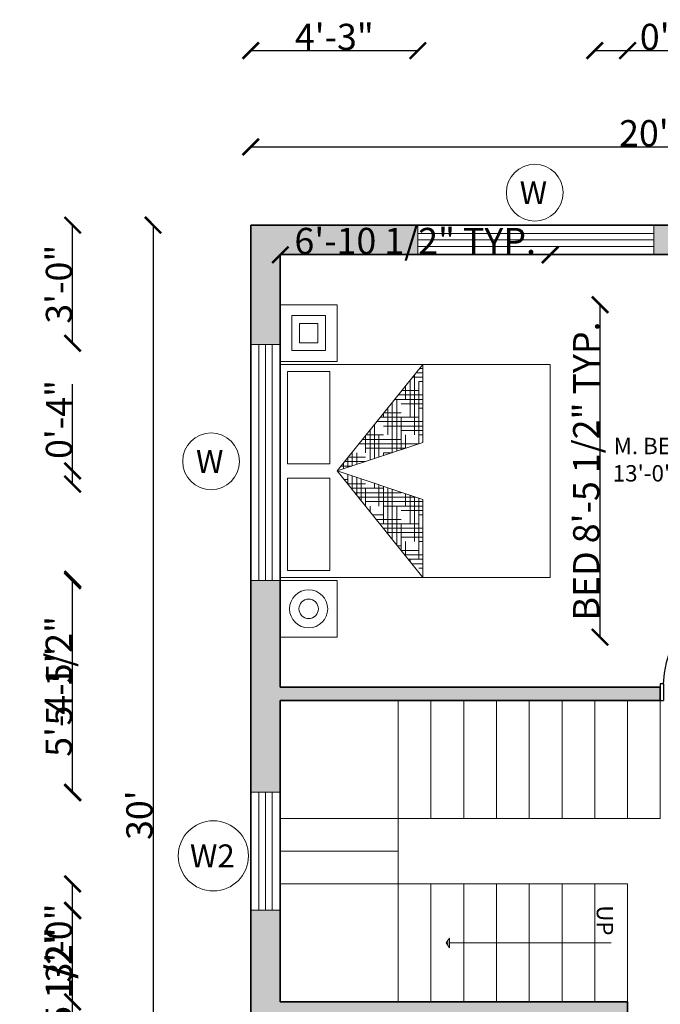
# Model space of a CAD drawing. Units: inches. Extents: x 2209 to 2954, y 1760 to 2265.
# Tile 3 of 7: x 2209 to 2404, y 1945 to 2245. Entities that reach past the tile are written whole.
import ezdxf

# ---------------------------------------------------------------- set-up
doc = ezdxf.new("R2010")
doc.units = ezdxf.units.IN
for name, color, linetype, lineweight in [('A-ANNO-DIMS', 2, 'Continuous', 18), ('A-ANNO-SYMB', 7, 'Continuous', 18), ('A-AREA-IDEN', 7, 'Continuous', 18), ('A-FURN', 8, 'Continuous', 18), ('A-WALL-PATT', 30, 'Continuous', 13), ('DOOR', 240, 'Continuous', 25), ('STEPS', 50, 'Continuous', 18), ('WALL', 7, 'Continuous', 35), ('WINDOW', 190, 'Continuous', 18)]:
    doc.layers.add(name, color=color, linetype=linetype, lineweight=lineweight)
doc.styles.get("Standard").update_dxf_attribs({"font": 'arial.ttf'})
doc.dimstyles.get("Standard").update_dxf_attribs({"dimtxt": 8, "dimasz": 5, "dimexe": 0.18, "dimexo": 0.0625, "dimgap": 0.09, "dimtad": 1, "dimdec": 1, "dimzin": 0, "dimdsep": 46, "dimlunit": 4, "dimtxsty": 'Standard', "dimblk": 'ARCHTICK', "dimcen": 0.09, "dimse1": 1, "dimse2": 1, "dimadec": 0, "dimazin": 0, "dimtfac": 1, "dimtdec": 1, "dimtofl": 0, "dimtmove": 0, "dimatfit": 3, "dimfxl": 1, "dimtolj": 1, "dimtzin": 0, "dimarcsym": 0})

# ---------------------------------------------------------------- blocks, each defined once
blk = doc.blocks.new('AP0B05')
for p, q in [((35, 100), (35, 880)), ((75, 100), (75, 878.9)), ((35, 100), (11, 100)), ((11, 100), (11, -20)), ((35, 100), (35, -20)), ((815, 100), (815, -20)), ((815, 100), (839, 100)), ((839, 100), (839, -20)), ((11, -20), (35, -20)), ((839, -20), (815, -20))]:
    blk.add_line(p, q)
blk.add_lwpolyline([(35, 100), (75, 100)])
blk.add_arc((-2.4, 62.6), 818.3, 2.62122, 87.37878)
blk = doc.blocks.new('*X3')
at = {"color": 0}
for p, q in [((20.1875, 14.75), (20.1875, 14.7669)), ((20.199, 14.7812), (20.2772, 14.7812)), ((20.25, 14.8125), (20.2772, 14.8125)), ((20.125, 14.5), (20.125, 14.6893)), ((20.1487, 14.7188), (20.2772, 14.7188)), ((20.1562, 14.625), (20.1562, 14.7281)), ((20.1739, 14.75), (20.2772, 14.75)), ((20.25, 14.3194), (20.25, 14.75)), ((20.0938, 14.375), (20.0938, 14.6504)), ((20.0984, 14.6562), (20.125, 14.6562)), ((20.1236, 14.6875), (20.25, 14.6875)), ((20.2188, 14.3091), (20.2188, 14.625)), ((20.25, 14.625), (20.2772, 14.625)), ((20.023, 14.5625), (20.2772, 14.5625)), ((20.0312, 14.2469), (20.0312, 14.5727)), ((20.0625, 14.2573), (20.0625, 14.6116)), ((20.125, 14.5938), (20.2772, 14.5938)), ((19.9727, 14.5), (20.25, 14.5)), ((19.9979, 14.5312), (20.2772, 14.5312)), ((20, 14.2366), (20, 14.5)), ((20.1875, 14.2987), (20.1875, 14.5)), ((19.9062, 14.375), (19.9062, 14.4174)), ((19.9225, 14.4375), (20, 14.4375)), ((19.9476, 14.4688), (20.125, 14.4688)), ((20.25, 14.4375), (20.2772, 14.4375)), ((19.875, 14.25), (19.875, 14.3785)), ((19.875, 14.3438), (20.2772, 14.3438)), ((19.9688, 14.2262), (19.9688, 14.375)), ((20, 14.375), (20.2772, 14.375)), ((20.125, 14.4062), (20.2772, 14.4062)), ((20.1562, 14.2884), (20.1562, 14.375)), ((19.7967, 14.2812), (20.125, 14.2812)), ((19.8125, 14.1744), (19.8125, 14.3008)), ((19.8219, 14.3125), (20.2291, 14.3125)), ((19.8438, 14.1848), (19.8438, 14.3397)), ((19.7465, 14.2188), (19.875, 14.2188)), ((19.75, 14.1537), (19.75, 14.2231)), ((19.7716, 14.25), (20, 14.25)), ((19.7812, 14.1641), (19.7812, 14.262)), ((19.9375, 14.2159), (19.9375, 14.25)), ((19.7213, 14.1875), (19.75, 14.1875)), ((19.7018, 14.0938), (19.7786, 14.0938)), ((19.7188, 14.0726), (19.7188, 14.1136)), ((19.75, 14.0338), (19.75, 14.1032)), ((19.7812, 13.9949), (19.7812, 14.0929)), ((19.8125, 14), (19.8125, 14.0825)), ((19.7269, 14.0625), (19.8728, 14.0625)), ((19.752, 14.0312), (19.875, 14.0312)), ((19.875, 13.8784), (19.875, 14)), ((19.9062, 13.8396), (19.9062, 14.0514)), ((19.9375, 13.8007), (19.9375, 14.0411)), ((19.9688, 13.875), (19.9688, 14.0307)), ((20, 14), (20, 14.0204)), ((20, 14), (20.0614, 14)), ((20.0625, 13.6454), (20.0625, 13.9996)), ((19.8275, 13.9375), (20.25, 13.9375)), ((19.875, 13.9688), (20.1557, 13.9688)), ((20.0938, 13.625), (20.0938, 13.9893)), ((20.125, 13.75), (20.125, 13.9789)), ((20.1562, 13.875), (20.1562, 13.9686)), ((20.25, 13.5), (20.25, 13.9375)), ((19.8526, 13.9062), (20.125, 13.9062)), ((19.8777, 13.875), (20, 13.875)), ((20.0312, 13.6842), (20.0312, 13.875)), ((20.2188, 13.4511), (20.2188, 13.875)), ((20.25, 13.875), (20.2772, 13.875)), ((20, 13.8125), (20.2772, 13.8125)), ((20.125, 13.8438), (20.2772, 13.8438)), ((19.9532, 13.7812), (20.2772, 13.7812)), ((19.9783, 13.75), (20.25, 13.75)), ((20, 13.723), (20, 13.75)), ((20.0035, 13.7188), (20.125, 13.7188)), ((20.1875, 13.49), (20.1875, 13.75)), ((20.125, 13.6562), (20.2772, 13.6562)), ((20.25, 13.6875), (20.2772, 13.6875)), ((20.0789, 13.625), (20.2772, 13.625)), ((20.104, 13.5938), (20.2772, 13.5938)), ((20.1562, 13.5288), (20.1562, 13.625)), ((20.1292, 13.5625), (20.25, 13.5625)), ((20.2046, 13.4688), (20.2772, 13.4688)), ((20.25, 13.5), (20.2772, 13.5)), ((20.2297, 13.4375), (20.2772, 13.4375)), ((20.2549, 13.4062), (20.2772, 13.4062))]:
    blk.add_line(p, q, dxfattribs=at)
blk = doc.blocks.new('MAT-P13')
for p, q in [((-1.17, 0), (-1.17, -0.4)), ((-1.17, 0), (-0.77, 0)), ((-0.77, 0), (-0.77, -0.4)), ((-0.75, 0), (0.75, 0)), ((-0.75, 0), (-0.75, -1.9)), ((0.75, 0), (0.75, -1.9)), ((0.77, 0), (1.17, 0)), ((0.77, 0), (0.77, -0.4)), ((1.17, 0), (1.17, -0.4)), ((-0.7, -0.05), (-0.7, -0.35)), ((-0.7, -0.05), (-0.05, -0.05)), ((-0.05, -0.35), (-0.05, -0.05)), ((0.05, -0.05), (0.7, -0.05)), ((0.05, -0.35), (0.05, -0.05)), ((0.7, -0.05), (0.7, -0.35)), ((-1.17, -0.4), (-0.77, -0.4)), ((-0.75, -1.0034), (0, -0.4)), ((0, -0.4), (-0.75, -1.0034)), ((-0.7, -0.35), (-0.05, -0.35)), ((0, -0.4), (-0.2, -1.0034)), ((0, -0.4), (0.2, -1.0034)), ((0, -0.4), (0.75, -1.0034)), ((0.05, -0.35), (0.7, -0.35)), ((0.77, -0.4), (1.17, -0.4)), ((-0.75, -1.0034), (-0.2, -1.0034)), ((0.2, -1.0034), (0.75, -1.0034)), ((0.75, -1.9), (-0.75, -1.9))]:
    blk.add_line(p, q)
for points in [[(0.8468, -0.0814), (1.0932, -0.0814), (1.0932, -0.3186), (0.8468, -0.3186)], [(0.9015, -0.1361), (1.0385, -0.1361), (1.0385, -0.2639), (0.9015, -0.2639)]]:
    blk.add_lwpolyline(points, close=True)
for radius in [0.1342, 0.0686]:
    blk.add_circle((-0.97, -0.2), radius)
at = {"xscale": -1, "rotation": 90}
blk.add_blockref('*X3', (14.1285, 19.2738), dxfattribs=at)
blk = doc.blocks.new('_ArchTick')
at = {"color": 0, "linetype": 'ByBlock', "const_width": 0.15}
blk.add_lwpolyline([(-0.5, -0.5), (0.5, 0.5)], dxfattribs=at)
blk = doc.blocks.new('*D13')
at = {"layer": 'A-ANNO-DIMS', "color": 0, "lineweight": -2, "transparency": 16777216}
blk.add_line((2279.15, 2206.17), (2519.15, 2206.17), dxfattribs=at)
at = {"layer": 'Defpoints', "color": 0, "transparency": 16777216}
for p in [(2519.15, 2206.17), (2279.15, 2182.29), (2519.15, 2182.29)]:
    blk.add_point(p, dxfattribs=at)
at = {"layer": 'A-ANNO-DIMS', "color": 0, "lineweight": -2, "transparency": 16777216, "xscale": 5, "yscale": 5, "zscale": 5, "rotation": 180}
blk.add_blockref('_ArchTick', (2279.15, 2206.17), dxfattribs=at)
at = {"layer": 'A-ANNO-DIMS', "color": 0, "lineweight": -2, "transparency": 16777216, "xscale": 5, "yscale": 5, "zscale": 5}
blk.add_blockref('_ArchTick', (2519.15, 2206.17), dxfattribs=at)
at = {"layer": 'A-ANNO-DIMS', "color": 0, "transparency": 16777216, "insert": (2399.15, 2210.34), "char_height": 8, "attachment_point": 5}
blk.add_mtext("\\A1;20'", dxfattribs=at)
blk = doc.blocks.new('*D14')
at = {"layer": 'A-ANNO-DIMS', "color": 0, "lineweight": -2, "transparency": 16777216}
blk.add_line((2249.34, 2182.29), (2249.34, 1822.29), dxfattribs=at)
at = {"layer": 'Defpoints', "color": 0, "transparency": 16777216}
for p in [(2279.15, 2182.29), (2249.34, 1822.29), (2279.15, 1822.29)]:
    blk.add_point(p, dxfattribs=at)
at = {"layer": 'A-ANNO-DIMS', "color": 0, "lineweight": -2, "transparency": 16777216, "xscale": 5, "yscale": 5, "zscale": 5}
for p, rotation in [((2249.34, 2182.29), 90), ((2249.34, 1822.29), 270)]:
    blk.add_blockref('_ArchTick', p, dxfattribs=dict(at, rotation=rotation))
at = {"layer": 'A-ANNO-DIMS', "color": 0, "transparency": 16777216, "insert": (2245.16, 2002.29), "char_height": 8, "attachment_point": 5, "rotation": 90}
blk.add_mtext("\\A1;30'", dxfattribs=at)
blk = doc.blocks.new('WIN-W-72IN')
for p, q in [((0, 6.5), (72, 6.5)), ((0, 4.5), (72, 4.5)), ((0, 2.5), (72, 2.5))]:
    blk.add_line(p, q)
blk.add_lwpolyline([(0, 9), (72, 9), (72, 0), (0, 0)], close=True)
blk = doc.blocks.new('WIN-W2-36IN')
for p, q in [((2.5, 0), (2.5, 36)), ((4.5, 0), (4.5, 36)), ((6.5, 0), (6.5, 36))]:
    blk.add_line(p, q)
blk.add_lwpolyline([(0, 0), (0, 36), (9, 36), (9, 0)], close=True)
blk = doc.blocks.new('STAIR-RETURN-36IN')
for p, q in [((36, 0), (36, 92)), ((46, 56), (46, 92)), ((56, 56), (56, 92)), ((66, 56), (66, 92)), ((76, 56), (76, 92)), ((86, 56), (86, 92)), ((96, 56), (96, 92)), ((106, 56), (106, 92)), ((116, 56), (116, 92)), ((116, 56), (0, 56)), ((36, 46), (0, 46)), ((106, 36), (0, 36)), ((46, 0), (46, 36)), ((56, 0), (56, 36)), ((66, 0), (66, 36)), ((76, 0), (76, 36)), ((86, 0), (86, 36)), ((96, 0), (96, 36)), ((106, 0), (106, 36))]:
    blk.add_line(p, q)
blk = doc.blocks.new('TAG-OPENING-W')
blk.add_circle((0, 0), 8.66)
blk.add_text('W', height=7).set_placement((-4.62, -3.5))
blk = doc.blocks.new('TAG-OPENING-W2')
blk.add_circle((0, 0), 10.71)
blk.add_text('W2', height=7).set_placement((-7.14, -3.51))
blk = doc.blocks.new('ARROW-STAIR-DIRECTION')
h = blk.add_hatch()
h.set_pattern_fill('ANGLE', color=256, angle=90)
h.set_pattern_definition([(90, (1948.154, -2410.884), (-6.985, 4e-16), [5.08, -1.905]), (180, (1948.154, -2410.884), (-9e-16, -6.985), [5.08, -1.905])])
h.paths.add_polyline_path([(0, 1.5), (1, 0), (1, 3)])
for p, q in [((0, 1.5), (1, 3)), ((0, 1.5), (1, 0)), ((1, 0), (1, 3)), ((50.28, 1.5), (1, 1.5))]:
    blk.add_line(p, q)
blk = doc.blocks.new('*D53')
at = {"layer": 'A-ANNO-DIMS', "color": 0, "lineweight": -2, "transparency": 16777216}
blk.add_line((2385.75, 2056.56), (2385.75, 2158.01), dxfattribs=at)
at = {"layer": 'Defpoints', "color": 0, "transparency": 16777216}
for p in [(2370.53, 2158.01), (2385.75, 2158.01), (2370.53, 2056.56)]:
    blk.add_point(p, dxfattribs=at)
at = {"layer": 'A-ANNO-DIMS', "color": 0, "lineweight": -2, "transparency": 16777216, "xscale": 5, "yscale": 5, "zscale": 5}
for p, rotation in [((2385.75, 2158.01), 90), ((2385.75, 2056.56), 270)]:
    blk.add_blockref('_ArchTick', p, dxfattribs=dict(at, rotation=rotation))
at = {"layer": 'A-ANNO-DIMS', "color": 0, "transparency": 16777216, "insert": (2381.53, 2107.29), "char_height": 8, "attachment_point": 5, "rotation": 90}
blk.add_mtext('\\A1;BED 8\'-5 1/2" TYP.', dxfattribs=at)
blk = doc.blocks.new('*D54')
at = {"layer": 'A-ANNO-DIMS', "color": 0, "lineweight": -2, "transparency": 16777216}
blk.add_line((2370.53, 2173.23), (2288.15, 2173.23), dxfattribs=at)
at = {"layer": 'Defpoints', "color": 0, "transparency": 16777216}
for p in [(2288.15, 2173.23), (2288.15, 2158.01), (2370.53, 2158.01)]:
    blk.add_point(p, dxfattribs=at)
at = {"layer": 'A-ANNO-DIMS', "color": 0, "lineweight": -2, "transparency": 16777216, "xscale": 5, "yscale": 5, "zscale": 5, "rotation": 180}
blk.add_blockref('_ArchTick', (2288.15, 2173.23), dxfattribs=at)
at = {"layer": 'A-ANNO-DIMS', "color": 0, "lineweight": -2, "transparency": 16777216, "xscale": 5, "yscale": 5, "zscale": 5}
blk.add_blockref('_ArchTick', (2370.53, 2173.23), dxfattribs=at)
at = {"layer": 'A-ANNO-DIMS', "color": 0, "transparency": 16777216, "insert": (2329.34, 2177.46), "char_height": 8, "attachment_point": 5}
blk.add_mtext('\\A1;6\'-10 1/2" TYP.', dxfattribs=at)
blk = doc.blocks.new('*D62')
at = {"layer": 'A-ANNO-DIMS', "color": 0, "lineweight": -2, "transparency": 16777216}
blk.add_line((2417.88, 1961.89), (2417.88, 2018.6), dxfattribs=at)
at = {"layer": 'Defpoints', "color": 0, "transparency": 16777216}
for p in [(2417.88, 2018.6), (2429.48, 2018.6), (2429.48, 1961.89)]:
    blk.add_point(p, dxfattribs=at)
at = {"layer": 'A-ANNO-DIMS', "color": 0, "lineweight": -2, "transparency": 16777216, "xscale": 5, "yscale": 5, "zscale": 5}
for p, rotation in [((2417.88, 2018.6), 90), ((2417.88, 1961.89), 270)]:
    blk.add_blockref('_ArchTick', p, dxfattribs=dict(at, rotation=rotation))
at = {"layer": 'A-ANNO-DIMS', "color": 0, "transparency": 16777216, "insert": (2413.65, 1990.24), "char_height": 8, "attachment_point": 5, "rotation": 90}
blk.add_mtext('\\A1;4\'-8 1/2"', dxfattribs=at)
blk = doc.blocks.new('*D70')
at = {"layer": 'A-ANNO-DIMS', "color": 0, "lineweight": -2, "transparency": 16777216}
blk.add_line((2279.15, 2235.55), (2330.15, 2235.55), dxfattribs=at)
at = {"layer": 'Defpoints', "color": 0, "transparency": 16777216}
for p in [(2330.15, 2235.55), (2279.15, 2182.29), (2330.15, 2182.29)]:
    blk.add_point(p, dxfattribs=at)
at = {"layer": 'A-ANNO-DIMS', "color": 0, "lineweight": -2, "transparency": 16777216, "xscale": 5, "yscale": 5, "zscale": 5, "rotation": 180}
blk.add_blockref('_ArchTick', (2279.15, 2235.55), dxfattribs=at)
at = {"layer": 'A-ANNO-DIMS', "color": 0, "lineweight": -2, "transparency": 16777216, "xscale": 5, "yscale": 5, "zscale": 5}
blk.add_blockref('_ArchTick', (2330.15, 2235.55), dxfattribs=at)
at = {"layer": 'A-ANNO-DIMS', "color": 0, "transparency": 16777216, "insert": (2304.65, 2239.73), "char_height": 8, "attachment_point": 5}
blk.add_mtext('\\A1;4\'-3"', dxfattribs=at)
blk = doc.blocks.new('*D72')
at = {"layer": 'A-ANNO-DIMS', "color": 0, "lineweight": -2, "transparency": 16777216}
blk.add_line((2224.78, 1919.97), (2224.78, 1973.29), dxfattribs=at)
at = {"layer": 'Defpoints', "color": 0, "transparency": 16777216}
for p in [(2224.78, 1973.29), (2279.15, 1973.29), (2279.15, 1919.97)]:
    blk.add_point(p, dxfattribs=at)
at = {"layer": 'A-ANNO-DIMS', "color": 0, "lineweight": -2, "transparency": 16777216, "xscale": 5, "yscale": 5, "zscale": 5}
for p, rotation in [((2224.78, 1973.29), 90), ((2224.78, 1919.97), 270)]:
    blk.add_blockref('_ArchTick', p, dxfattribs=dict(at, rotation=rotation))
at = {"layer": 'A-ANNO-DIMS', "color": 0, "transparency": 16777216, "insert": (2220.55, 1946.63), "char_height": 8, "attachment_point": 5, "rotation": 90}
blk.add_mtext('\\A1;4\'-5 1/2"', dxfattribs=at)
blk = doc.blocks.new('*D73')
at = {"layer": 'A-ANNO-DIMS', "color": 0, "lineweight": -2, "transparency": 16777216}
blk.add_line((2224.78, 2009.29), (2224.78, 2073.83), dxfattribs=at)
at = {"layer": 'Defpoints', "color": 0, "transparency": 16777216}
for p in [(2224.78, 2073.83), (2279.15, 2073.83), (2279.15, 2009.29)]:
    blk.add_point(p, dxfattribs=at)
at = {"layer": 'A-ANNO-DIMS', "color": 0, "lineweight": -2, "transparency": 16777216, "xscale": 5, "yscale": 5, "zscale": 5}
for p, rotation in [((2224.78, 2073.83), 90), ((2224.78, 2009.29), 270)]:
    blk.add_blockref('_ArchTick', p, dxfattribs=dict(at, rotation=rotation))
at = {"layer": 'A-ANNO-DIMS', "color": 0, "transparency": 16777216, "insert": (2220.55, 2041.56), "char_height": 8, "attachment_point": 5, "rotation": 90}
blk.add_mtext('\\A1;5\'-4 1/2"', dxfattribs=at)
blk = doc.blocks.new('*D78')
at = {"layer": 'A-ANNO-DIMS', "color": 0, "lineweight": -2, "transparency": 16777216}
blk.add_line((2224.78, 1945.29), (2224.78, 1981.29), dxfattribs=at)
at = {"layer": 'Defpoints', "color": 0, "transparency": 16777216}
for p in [(2224.78, 1981.29), (2288.15, 1981.29), (2288.15, 1945.29)]:
    blk.add_point(p, dxfattribs=at)
at = {"layer": 'A-ANNO-DIMS', "color": 0, "lineweight": -2, "transparency": 16777216, "xscale": 5, "yscale": 5, "zscale": 5}
for p, rotation in [((2224.78, 1981.29), 90), ((2224.78, 1945.29), 270)]:
    blk.add_blockref('_ArchTick', p, dxfattribs=dict(at, rotation=rotation))
at = {"layer": 'A-ANNO-DIMS', "color": 0, "transparency": 16777216, "insert": (2220.6, 1963.29), "char_height": 8, "attachment_point": 5, "rotation": 90}
blk.add_mtext('\\A1;3\'-0"', dxfattribs=at)
blk = doc.blocks.new('*D79')
at = {"layer": 'A-ANNO-DIMS', "color": 0, "lineweight": -2, "transparency": 16777216}
for p, q in [((2384.15, 2235.55), (2394.15, 2235.55)), ((2394.15, 2235.55), (2426.82, 2235.55))]:
    blk.add_line(p, q, dxfattribs=at)
at = {"layer": 'Defpoints', "color": 0, "transparency": 16777216}
for p in [(2394.15, 2235.55), (2384.15, 1981.29), (2394.15, 1981.29)]:
    blk.add_point(p, dxfattribs=at)
at = {"layer": 'A-ANNO-DIMS', "color": 0, "lineweight": -2, "transparency": 16777216, "xscale": 5, "yscale": 5, "zscale": 5, "rotation": 180}
blk.add_blockref('_ArchTick', (2384.15, 2235.55), dxfattribs=at)
at = {"layer": 'A-ANNO-DIMS', "color": 0, "lineweight": -2, "transparency": 16777216, "xscale": 5, "yscale": 5, "zscale": 5}
blk.add_blockref('_ArchTick', (2394.15, 2235.55), dxfattribs=at)
at = {"layer": 'A-ANNO-DIMS', "color": 0, "transparency": 16777216, "insert": (2412.99, 2239.72), "char_height": 8, "attachment_point": 5}
blk.add_mtext('\\A1;0\'-10"', dxfattribs=at)
blk = doc.blocks.new('*D87')
at = {"layer": 'A-ANNO-DIMS', "color": 0, "lineweight": -2, "transparency": 16777216}
blk.add_line((2224.78, 2146.27), (2224.78, 2182.29), dxfattribs=at)
at = {"layer": 'Defpoints', "color": 0, "transparency": 16777216}
for p in [(2224.78, 2182.29), (2629.22, 2182.29), (2629.22, 2146.27)]:
    blk.add_point(p, dxfattribs=at)
at = {"layer": 'A-ANNO-DIMS', "color": 0, "lineweight": -2, "transparency": 16777216, "xscale": 5, "yscale": 5, "zscale": 5}
for p, rotation in [((2224.78, 2182.29), 90), ((2224.78, 2146.27), 270)]:
    blk.add_blockref('_ArchTick', p, dxfattribs=dict(at, rotation=rotation))
at = {"layer": 'A-ANNO-DIMS', "color": 0, "transparency": 16777216, "insert": (2220.6, 2164.28), "char_height": 8, "attachment_point": 5, "rotation": 90}
blk.add_mtext('\\A1;3\'-0"', dxfattribs=at)
blk = doc.blocks.new('*D88')
at = {"layer": 'A-ANNO-DIMS', "color": 0, "lineweight": -2, "transparency": 16777216}
blk.add_line((2224.78, 1919.53), (2224.78, 1973.14), dxfattribs=at)
at = {"layer": 'Defpoints', "color": 0, "transparency": 16777216}
for p in [(2224.78, 1973.14), (2629.22, 1973.14), (2629.22, 1919.53)]:
    blk.add_point(p, dxfattribs=at)
at = {"layer": 'A-ANNO-DIMS', "color": 0, "lineweight": -2, "transparency": 16777216, "xscale": 5, "yscale": 5, "zscale": 5}
for p, rotation in [((2224.78, 1973.14), 90), ((2224.78, 1919.53), 270)]:
    blk.add_blockref('_ArchTick', p, dxfattribs=dict(at, rotation=rotation))
at = {"layer": 'A-ANNO-DIMS', "color": 0, "transparency": 16777216, "insert": (2220.55, 1946.34), "char_height": 8, "attachment_point": 5, "rotation": 90}
blk.add_mtext('\\A1;4\'-5 1/2"', dxfattribs=at)
blk = doc.blocks.new('*D89')
at = {"layer": 'A-ANNO-DIMS', "color": 0, "lineweight": -2, "transparency": 16777216}
blk.add_line((2224.78, 2009.14), (2224.78, 2074.27), dxfattribs=at)
at = {"layer": 'Defpoints', "color": 0, "transparency": 16777216}
for p in [(2224.78, 2074.27), (2629.22, 2074.27), (2629.22, 2009.14)]:
    blk.add_point(p, dxfattribs=at)
at = {"layer": 'A-ANNO-DIMS', "color": 0, "lineweight": -2, "transparency": 16777216, "xscale": 5, "yscale": 5, "zscale": 5}
for p, rotation in [((2224.78, 2074.27), 90), ((2224.78, 2009.14), 270)]:
    blk.add_blockref('_ArchTick', p, dxfattribs=dict(at, rotation=rotation))
at = {"layer": 'A-ANNO-DIMS', "color": 0, "transparency": 16777216, "insert": (2220.62, 2041.7), "char_height": 8, "attachment_point": 5, "rotation": 90}
blk.add_mtext('\\A1;5\'-5"', dxfattribs=at)
blk = doc.blocks.new('*D93')
at = {"layer": 'A-ANNO-DIMS', "color": 0, "lineweight": -2, "transparency": 16777216}
for p, q in [((2224.78, 2107.29), (2224.78, 2133.73)), ((2224.78, 2103.29), (2224.78, 2107.29))]:
    blk.add_line(p, q, dxfattribs=at)
at = {"layer": 'Defpoints', "color": 0, "transparency": 16777216}
for p in [(2224.78, 2107.29), (2798.22, 2107.29), (2798.22, 2103.29)]:
    blk.add_point(p, dxfattribs=at)
at = {"layer": 'A-ANNO-DIMS', "color": 0, "lineweight": -2, "transparency": 16777216, "xscale": 5, "yscale": 5, "zscale": 5}
for p, rotation in [((2224.78, 2107.29), 90), ((2224.78, 2103.29), 270)]:
    blk.add_blockref('_ArchTick', p, dxfattribs=dict(at, rotation=rotation))
at = {"layer": 'A-ANNO-DIMS', "color": 0, "transparency": 16777216, "insert": (2220.61, 2123.01), "char_height": 8, "attachment_point": 5, "rotation": 90}
blk.add_mtext('\\A1;0\'-4"', dxfattribs=at)

msp = doc.modelspace()

# ---------------------------------------------------------------- hatches: boundary and pattern name
at = {"layer": 'A-WALL-PATT', "transparency": 33554585}
h = msp.add_hatch(color=256, dxfattribs=at)
h.dxf.hatch_style = 1
h.paths.add_polyline_path([(2519.15, 2182.29), (2402.15, 2182.29), (2402.15, 2173.29), (2444.15, 2173.29), (2444.15, 2154.12), (2448.15, 2154.12), (2448.15, 2173.29), (2510.15, 2173.29), (2510.15, 2167.29), (2519.15, 2167.29)])
h.paths.add_polyline_path([(2330.15, 2182.29), (2279.15, 2182.29), (2279.15, 2145.83), (2288.15, 2145.83), (2288.15, 2158.01), (2288.15, 2173.29), (2330.15, 2173.29)])
h.paths.add_polyline_path([(2288.15, 2073.83), (2279.15, 2073.83), (2279.15, 2009.29), (2288.15, 2009.29), (2288.15, 2037.29), (2404.15, 2037.29), (2404.15, 2041.29), (2288.15, 2041.29)])
h.paths.add_polyline_path([(2519.15, 2131.29), (2510.15, 2131.29), (2510.15, 2125.29), (2444.15, 2125.29), (2444.15, 2041.29), (2439.11, 2041.29), (2439.11, 2037.29), (2448.15, 2037.29), (2448.15, 2069.29), (2481.65, 2069.29), (2481.65, 2073.29), (2448.15, 2073.29), (2448.15, 2121.29), (2468.19, 2121.29), (2468.19, 2121.32), (2488.37, 2121.32), (2510.15, 2121.29), (2510.15, 2113.63), (2519.15, 2113.63)])
h.paths.add_polyline_path([(2519.15, 2077.63), (2510.15, 2077.63), (2510.15, 2073.32), (2510.17, 2073.32), (2510.15, 2069.19), (2510.15, 2043.25), (2519.15, 2043.25)], flags=17)
h.paths.add_polyline_path([(2519.15, 1971.25), (2510.15, 1971.25), (2510.15, 1945.29), (2444.15, 1945.29), (2444.15, 1937.21), (2448.15, 1937.21), (2448.15, 1941.29), (2510.15, 1941.29), (2510.15, 1922.29), (2519.15, 1922.29)])
h.paths.add_polyline_path([(2288.15, 1941.29), (2394.15, 1941.29), (2394.15, 1945.29), (2288.15, 1945.29), (2288.15, 1973.29), (2279.15, 1973.29), (2279.15, 1919.97), (2288.15, 1919.97)])
h.paths.add_polyline_path([(2300.65, 1831.29), (2288.15, 1831.29), (2288.15, 1847.97), (2279.15, 1847.97), (2279.15, 1822.29), (2300.65, 1822.29)])
h.paths.add_polyline_path([(2394.15, 1825.29), (2394.15, 1831.29), (2372.65, 1831.29), (2372.65, 1822.29), (2394.15, 1822.29)])
h.paths.add_polyline_path([(2449.17, 1831.29), (2448.15, 1831.29), (2448.15, 1899.32), (2444.15, 1899.32), (2444.15, 1831.29), (2439.18, 1831.29), (2439.18, 1822.29), (2449.17, 1822.29)])
h.paths.add_polyline_path([(2519.15, 1850.29), (2510.15, 1850.29), (2510.15, 1831.29), (2509.17, 1831.29), (2509.17, 1822.29), (2519.15, 1822.29)])
h.paths.add_polyline_path([(2638.22, 1941.29), (2744.22, 1941.29), (2744.22, 1945.29), (2638.22, 1945.29), (2638.22, 1973.14), (2629.22, 1973.14), (2629.22, 1919.53), (2638.22, 1919.53)])
h.paths.add_polyline_path([(2638.22, 1847.53), (2629.22, 1847.53), (2629.22, 1822.29), (2650.72, 1822.29), (2650.72, 1831.29), (2638.22, 1831.29)])
h.paths.add_polyline_path([(2638.22, 2037.29), (2754.22, 2037.29), (2754.22, 2041.29), (2638.22, 2041.29), (2638.22, 2074.27), (2629.22, 2074.27), (2629.22, 2009.14), (2638.22, 2009.14)])
h.paths.add_polyline_path([(2803.22, 1936.29), (2812.78, 1936.29), (2812.78, 1945.29), (2791.22, 1945.29), (2791.22, 1936.29), (2794.22, 1936.29), (2794.22, 1831.29), (2722.72, 1831.29), (2722.72, 1822.29), (2803.22, 1822.29)])
h.paths.add_polyline_path([(2869.22, 1955.43), (2860.22, 1955.43), (2860.22, 1945.29), (2853.36, 1945.29), (2853.36, 1936.29), (2869.22, 1936.29)])
h.paths.add_polyline_path([(2680.22, 2182.29), (2629.22, 2182.29), (2629.22, 2146.27), (2638.22, 2146.27), (2638.22, 2173.29), (2680.22, 2173.29)])
h.paths.add_polyline_path([(2869.22, 2182.29), (2752.22, 2182.29), (2752.22, 2173.29), (2794.22, 2173.29), (2794.22, 2142.92), (2798.22, 2142.92), (2798.22, 2173.29), (2860.22, 2173.29), (2860.22, 2158.46), (2869.22, 2158.46)])
h.paths.add_polyline_path([(2869.22, 2122.46), (2860.22, 2122.46), (2860.22, 2090.29), (2869.22, 2090.29)])

# ---------------------------------------------------------------- linework, layer by layer
at = {"layer": 'WALL'}
for p, q in [((2279.15, 2182.29), (2519.15, 2182.29)), ((2279.15, 2182.29), (2279.15, 1822.29)), ((2288.15, 2173.29), (2444.15, 2173.29)), ((2288.15, 2173.29), (2288.15, 2041.29)), ((2288.15, 2041.29), (2404.15, 2041.29)), ((2404.15, 2037.29), (2404.15, 2041.29)), ((2288.15, 2037.29), (2404.15, 2037.29)), ((2288.15, 2037.29), (2288.15, 1945.29)), ((2288.15, 1945.29), (2394.15, 1945.29)), ((2394.15, 1945.29), (2394.15, 1941.29))]:
    msp.add_line(p, q, dxfattribs=at)

# ---------------------------------------------------------------- block references
at = {"layer": 'A-ANNO-SYMB'}
for name, p in [('TAG-OPENING-W', (2365.84, 2192.21)), ('TAG-OPENING-W', (2267.05, 2110.22)), ('TAG-OPENING-W2', (2267.73, 1989.86)), ('ARROW-STAIR-DIRECTION', (2338.84, 1961.79))]:
    msp.add_blockref(name, p, dxfattribs=at)
at = {"layer": 'A-FURN', "xscale": 43.35755422729858, "yscale": 43.35755422729858, "zscale": 43.35755422729858, "rotation": 90}
msp.add_blockref('MAT-P13', (2288.15, 2107.29), dxfattribs=at)
at = {"layer": 'DOOR', "xscale": -0.0422149343000146, "yscale": 0.0422149343000146, "zscale": 0.0422149343000146}
msp.add_blockref('AP0B05', (2439.57, 2038.13), dxfattribs=at)
at = {"layer": 'STEPS'}
msp.add_blockref('STAIR-RETURN-36IN', (2288.15, 1945.29), dxfattribs=at)
at = {"layer": 'WINDOW'}
for name, p in [('WIN-W-72IN', (2330.15, 2173.29)), ('WIN-W2-36IN', (2279.15, 1973.29))]:
    msp.add_blockref(name, p, dxfattribs=at)
at = {"layer": 'WINDOW', "rotation": 89.99999999999984}
msp.add_blockref('WIN-W-72IN', (2288.15, 2073.83), dxfattribs=at)

# ---------------------------------------------------------------- texts
at = {"layer": 'A-ANNO-SYMB'}
msp.add_text('UP', height=5, rotation=270, dxfattribs=at).set_placement((2384.75, 1974.79))
at = {"layer": 'A-AREA-IDEN', "insert": (2388.44, 2117.41), "char_height": 5, "attachment_point": 1}
msp.add_mtext_dynamic_manual_height_columns("\\pxqc;M. BEDROOM\\P13'-0''X11'-0''", width=45.1409, gutter_width=12.5, heights=[0], dxfattribs=at)

# ---------------------------------------------------------------- dimensions: what is measured, and where the dimension line sits
at = {"layer": 'A-ANNO-DIMS'}
for base, p1, p2, override, picture, middle in [((2330.15, 2235.55), (2279.15, 2182.29), (2330.15, 2182.29), {"dimdec": 1, "dimlfac": 1, "dimrnd": 0, "dimzin": 1, "dimdsep": 46, "dimlunit": 4, "dimfrac": 2}, '*D70', (2304.65, 2239.73)), ((2394.15, 2235.55), (2384.15, 1981.29), (2394.15, 1981.29), {"dimdec": 1, "dimlfac": 1, "dimrnd": 0, "dimzin": 1, "dimdsep": 46, "dimlunit": 4, "dimfrac": 2}, '*D79', (2412.99, 2239.72)), ((2519.15, 2206.17), (2279.15, 2182.29), (2519.15, 2182.29), {"dimclrd": 0, "dimclre": 0, "dimclrt": 0}, '*D13', (2399.15, 2210.34))]:
    dim = msp.add_linear_dim(base=base, p1=p1, p2=p2, dimstyle='Standard', override=override, dxfattribs=at)
    dim.commit()
    dim.dimension.update_dxf_attribs({"geometry": picture, "text_midpoint": middle})
for base, p1, p2, angle, text, picture, middle in [((2288.15, 2173.23), (2370.53, 2158.01), (2288.15, 2158.01), 180, '<> TYP.', '*D54', (2329.34, 2177.46)), ((2385.7523, 2158.0135), (2370.5338, 2056.5568), (2370.5338, 2158.0135), 90, 'BED <> TYP.', '*D53', (2381.5259, 2107.2851))]:
    dim = msp.add_linear_dim(base=base, p1=p1, p2=p2, angle=angle, text=text, dimstyle='Standard', override={"dimdec": 1, "dimlfac": 1, "dimrnd": 0, "dimzin": 1, "dimdsep": 46, "dimlunit": 4, "dimfrac": 2}, dxfattribs=at)
    dim.commit()
    dim.dimension.update_dxf_attribs({"geometry": picture, "text_midpoint": middle})
for base, p1, p2, override, picture, middle in [((2224.78, 2182.29), (2629.22, 2146.27), (2629.22, 2182.29), {"dimdec": 1, "dimlfac": 1, "dimrnd": 0, "dimzin": 1, "dimdsep": 46, "dimlunit": 4, "dimfrac": 2}, '*D87', (2220.6, 2164.28)), ((2249.34, 1822.29), (2279.15, 2182.29), (2279.15, 1822.29), {"dimclrd": 0, "dimclre": 0, "dimclrt": 0}, '*D14', (2245.16, 2002.29)), ((2224.78, 2107.29), (2798.22, 2103.29), (2798.22, 2107.29), {"dimdec": 1, "dimlfac": 1, "dimrnd": 0, "dimzin": 1, "dimdsep": 46, "dimlunit": 4, "dimfrac": 2}, '*D93', (2220.61, 2123.01)), ((2224.78, 2073.83), (2279.15, 2009.29), (2279.15, 2073.83), {"dimdec": 1, "dimlfac": 1, "dimrnd": 0, "dimzin": 1, "dimdsep": 46, "dimlunit": 4, "dimfrac": 2}, '*D73', (2220.55, 2041.56)), ((2224.78, 2074.27), (2629.22, 2009.14), (2629.22, 2074.27), {"dimdec": 1, "dimlfac": 1, "dimrnd": 0, "dimzin": 1, "dimdsep": 46, "dimlunit": 4, "dimfrac": 2}, '*D89', (2220.62, 2041.7)), ((2417.88, 2018.6), (2429.48, 1961.89), (2429.48, 2018.6), {"dimdec": 1, "dimlfac": 1, "dimrnd": 0, "dimzin": 1, "dimdsep": 46, "dimlunit": 4, "dimfrac": 2}, '*D62', (2413.65, 1990.24)), ((2224.78, 1981.29), (2288.15, 1945.29), (2288.15, 1981.29), {"dimdec": 1, "dimlfac": 1, "dimrnd": 0, "dimzin": 1, "dimdsep": 46, "dimlunit": 4, "dimfrac": 2}, '*D78', (2220.6, 1963.29)), ((2224.78, 1973.29), (2279.15, 1919.97), (2279.15, 1973.29), {"dimdec": 1, "dimlfac": 1, "dimrnd": 0, "dimzin": 1, "dimdsep": 46, "dimlunit": 4, "dimfrac": 2}, '*D72', (2220.55, 1946.63)), ((2224.78, 1973.14), (2629.22, 1919.53), (2629.22, 1973.14), {"dimdec": 1, "dimlfac": 1, "dimrnd": 0, "dimzin": 1, "dimdsep": 46, "dimlunit": 4, "dimfrac": 2}, '*D88', (2220.55, 1946.34))]:
    dim = msp.add_linear_dim(base=base, p1=p1, p2=p2, angle=90, dimstyle='Standard', override=override, dxfattribs=at)
    dim.commit()
    dim.dimension.update_dxf_attribs({"geometry": picture, "text_midpoint": middle})

doc.saveas('drawing.dxf')
